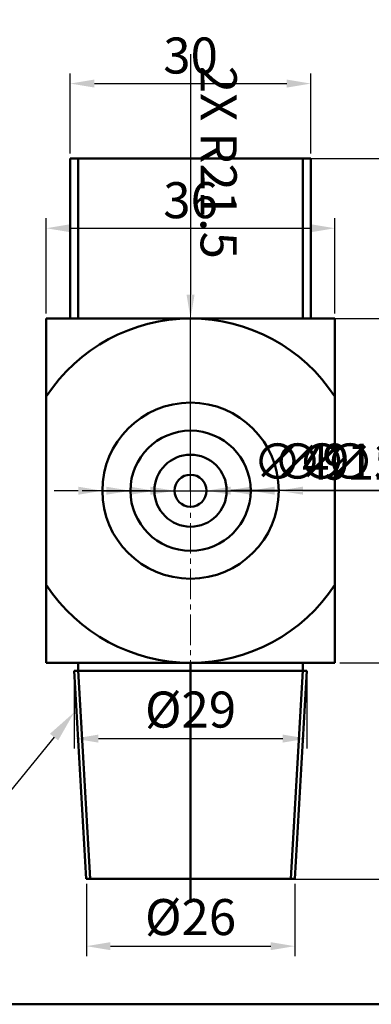
# Model space of a CAD drawing. Units: millimetres. Extents: x 418 to 773, y -46 to 294.
# Tile 3 of 7: x 565 to 609, y -46 to 77. Entities that reach past the tile are written whole.
import ezdxf
from ezdxf import colors
from ezdxf.entities.mleader import LeaderData, LeaderLine
from ezdxf.math import Vec2, Vec3

# ---------------------------------------------------------------- set-up
doc = ezdxf.new("R2010")
doc.units = ezdxf.units.MM
doc.header["$LTSCALE"] = 0.2
doc.linetypes.add('CENTER2', pattern=[28.575, 19.05, -3.175, 3.175, -3.175])
for name, color, linetype, lineweight in [('M-CNTR', 1, 'CENTER2', 18), ('M-DIMS', 2, 'Continuous', 25), ('M-OUTL', 7, 'Continuous', 50), ('M-TEXT', 3, 'Continuous', 25), ('M-TTLB', 7, 'Continuous', 50)]:
    doc.layers.add(name, color=color, linetype=linetype, lineweight=lineweight)
doc.styles.get("Standard").update_dxf_attribs({"font": 'arial.ttf'})
doc.dimstyles.new('ISO-25', dxfattribs={"dimtxt": 4.5, "dimasz": 3, "dimexe": 1.25, "dimexo": 0.625, "dimtad": 1, "dimdec": 1, "dimtxsty": 'Standard', "dimcen": 2.5, "dimadec": 0, "dimazin": 0, "dimtfac": 1, "dimtdec": 1, "dimtmove": 0, "dimatfit": 3, "dimfxl": 1, "dimarcsym": 0})

# ---------------------------------------------------------------- blocks, each defined once
blk = doc.blocks.new('*D87')
at = {"layer": 'Defpoints', "color": 0, "ltscale": 0.2, "transparency": 16777216}
for p in [(601.02, 68.54), (571.02, 59.18), (601.02, 59.18)]:
    blk.add_point(p, dxfattribs=at)
at = {"layer": 'M-DIMS', "color": 0, "lineweight": -2, "ltscale": 0.2, "transparency": 16777216}
for p, q in [((571.02, 59.81), (571.02, 69.79)), ((601.02, 59.81), (601.02, 69.79)), ((574.02, 68.54), (598.02, 68.54))]:
    blk.add_line(p, q, dxfattribs=at)
at = {"layer": 'M-DIMS', "color": 0, "ltscale": 0.2, "transparency": 16777216}
for points in [[(574.02, 69.04), (574.02, 68.04), (571.02, 68.54)], [(598.02, 69.04), (598.02, 68.04), (601.02, 68.54)]]:
    blk.add_solid(points, dxfattribs=at)
at = {"layer": 'M-DIMS', "color": 0, "ltscale": 0.2, "transparency": 16777216, "insert": (586.02, 71.46), "char_height": 4.5, "attachment_point": 5}
blk.add_mtext('30', dxfattribs=at)
blk = doc.blocks.new('*D88')
at = {"layer": 'Defpoints', "color": 0, "ltscale": 0.2, "transparency": 16777216}
for p in [(604.02, 50.47), (568.02, 39.18), (604.02, 39.18)]:
    blk.add_point(p, dxfattribs=at)
at = {"layer": 'M-DIMS', "color": 0, "lineweight": -2, "ltscale": 0.2, "transparency": 16777216}
for p, q in [((568.02, 39.81), (568.02, 51.72)), ((604.02, 39.81), (604.02, 51.72)), ((571.02, 50.47), (601.02, 50.47))]:
    blk.add_line(p, q, dxfattribs=at)
at = {"layer": 'M-DIMS', "color": 0, "ltscale": 0.2, "transparency": 16777216}
for points in [[(571.02, 50.97), (571.02, 49.97), (568.02, 50.47)], [(601.02, 50.97), (601.02, 49.97), (604.02, 50.47)]]:
    blk.add_solid(points, dxfattribs=at)
at = {"layer": 'M-DIMS', "color": 0, "ltscale": 0.2, "transparency": 16777216, "insert": (586.02, 53.39), "char_height": 4.5, "attachment_point": 5}
blk.add_mtext('36', dxfattribs=at)
blk = doc.blocks.new('*D90')
at = {"layer": 'Defpoints', "color": 0, "ltscale": 0.2, "transparency": 16777216}
for p in [(600.02, 59.18), (601.02, 39.18), (620.1, 39.18)]:
    blk.add_point(p, dxfattribs=at)
at = {"layer": 'M-DIMS', "color": 0, "lineweight": -2, "ltscale": 0.2, "transparency": 16777216}
for p, q in [((600.64, 59.18), (621.35, 59.18)), ((620.1, 56.18), (620.1, 42.18)), ((601.64, 39.18), (621.35, 39.18))]:
    blk.add_line(p, q, dxfattribs=at)
at = {"layer": 'M-DIMS', "color": 0, "ltscale": 0.2, "transparency": 16777216}
for points in [[(619.6, 56.18), (620.6, 56.18), (620.1, 59.18)], [(619.6, 42.18), (620.6, 42.18), (620.1, 39.18)]]:
    blk.add_solid(points, dxfattribs=at)
at = {"layer": 'M-DIMS', "color": 0, "ltscale": 0.2, "transparency": 16777216, "insert": (617.18, 49.18), "char_height": 4.5, "attachment_point": 5, "rotation": 90}
blk.add_mtext('20', dxfattribs=at)
blk = doc.blocks.new('*D91')
at = {"layer": 'Defpoints', "color": 0, "ltscale": 0.2, "transparency": 16777216}
for p in [(611.5, 39.18), (604.02, -3.82), (620.1, -3.82)]:
    blk.add_point(p, dxfattribs=at)
at = {"layer": 'M-DIMS', "color": 0, "lineweight": -2, "ltscale": 0.2, "transparency": 16777216}
for p, q in [((612.12, 39.18), (621.35, 39.18)), ((620.1, 36.18), (620.1, -0.82)), ((604.64, -3.82), (621.35, -3.82))]:
    blk.add_line(p, q, dxfattribs=at)
at = {"layer": 'M-DIMS', "color": 0, "ltscale": 0.2, "transparency": 16777216}
for points in [[(619.6, 36.18), (620.6, 36.18), (620.1, 39.18)], [(619.6, -0.82), (620.6, -0.82), (620.1, -3.82)]]:
    blk.add_solid(points, dxfattribs=at)
at = {"layer": 'M-DIMS', "color": 0, "ltscale": 0.2, "transparency": 16777216, "insert": (617.18, 17.68), "char_height": 4.5, "attachment_point": 5, "rotation": 90}
blk.add_mtext('43', dxfattribs=at)
blk = doc.blocks.new('*D92')
at = {"layer": 'Defpoints', "color": 0, "ltscale": 0.2, "transparency": 16777216}
for p in [(608.93, -3.82), (592.52, -30.82), (620.1, -30.82)]:
    blk.add_point(p, dxfattribs=at)
at = {"layer": 'M-DIMS', "color": 0, "lineweight": -2, "ltscale": 0.2, "transparency": 16777216}
for p, q in [((609.56, -3.82), (621.35, -3.82)), ((620.1, -6.82), (620.1, -27.82)), ((593.14, -30.82), (621.35, -30.82))]:
    blk.add_line(p, q, dxfattribs=at)
at = {"layer": 'M-DIMS', "color": 0, "ltscale": 0.2, "transparency": 16777216}
for points in [[(619.6, -6.82), (620.6, -6.82), (620.1, -3.82)], [(619.6, -27.82), (620.6, -27.82), (620.1, -30.82)]]:
    blk.add_solid(points, dxfattribs=at)
at = {"layer": 'M-DIMS', "color": 0, "ltscale": 0.2, "transparency": 16777216, "insert": (617.22, -17.32), "char_height": 4.5, "attachment_point": 5, "rotation": 90}
blk.add_mtext('27', dxfattribs=at)
blk = doc.blocks.new('*D93')
at = {"layer": 'Defpoints', "color": 0, "ltscale": 0.2, "transparency": 16777216}
for p in [(571.52, -4.82), (600.52, -4.82), (600.52, -13.28)]:
    blk.add_point(p, dxfattribs=at)
at = {"layer": 'M-DIMS', "color": 0, "lineweight": -2, "ltscale": 0.2, "transparency": 16777216}
for p, q in [((571.52, -5.44), (571.52, -14.53)), ((600.52, -5.44), (600.52, -14.53)), ((574.52, -13.28), (597.52, -13.28))]:
    blk.add_line(p, q, dxfattribs=at)
at = {"layer": 'M-DIMS', "color": 0, "ltscale": 0.2, "transparency": 16777216}
for points in [[(574.52, -12.78), (574.52, -13.78), (571.52, -13.28)], [(597.52, -12.78), (597.52, -13.78), (600.52, -13.28)]]:
    blk.add_solid(points, dxfattribs=at)
at = {"layer": 'M-DIMS', "color": 0, "ltscale": 0.2, "transparency": 16777216, "insert": (586.02, -10.24), "char_height": 4.5, "attachment_point": 5}
blk.add_mtext('%%C29', dxfattribs=at)
blk = doc.blocks.new('*D94')
at = {"layer": 'Defpoints', "color": 0, "ltscale": 0.2, "transparency": 16777216}
for p in [(573.02, -30.82), (599.02, -30.82), (599.02, -39.21)]:
    blk.add_point(p, dxfattribs=at)
at = {"layer": 'M-DIMS', "color": 0, "lineweight": -2, "ltscale": 0.2, "transparency": 16777216}
for p, q in [((573.02, -31.44), (573.02, -40.46)), ((599.02, -31.44), (599.02, -40.46)), ((576.02, -39.21), (596.02, -39.21))]:
    blk.add_line(p, q, dxfattribs=at)
at = {"layer": 'M-DIMS', "color": 0, "ltscale": 0.2, "transparency": 16777216}
for points in [[(576.02, -38.71), (576.02, -39.71), (573.02, -39.21)], [(596.02, -38.71), (596.02, -39.71), (599.02, -39.21)]]:
    blk.add_solid(points, dxfattribs=at)
at = {"layer": 'M-DIMS', "color": 0, "ltscale": 0.2, "transparency": 16777216, "insert": (586.02, -36.16), "char_height": 4.5, "attachment_point": 5}
blk.add_mtext('%%C26', dxfattribs=at)
blk = doc.blocks.new('*U95')
at = {"layer": 'M-CNTR', "color": 0, "transparency": 16777216}
blk.add_line((0, -25), (0, 47.23), dxfattribs=at)
blk = doc.blocks.new('*D101')
at = {"layer": 'Defpoints', "color": 0, "ltscale": 0.2, "transparency": 16777216}
for p in [(586.02, 39.18), (586.02, 17.68)]:
    blk.add_point(p, dxfattribs=at)
at = {"layer": 'M-DIMS', "color": 0, "lineweight": -2, "ltscale": 0.2, "transparency": 16777216}
for p, q in [((586.02, 72.21), (586.02, 42.18)), ((586.02, 17.68), (586.02, 39.18))]:
    blk.add_line(p, q, dxfattribs=at)
at = {"layer": 'M-DIMS', "color": 0, "ltscale": 0.2, "transparency": 16777216}
blk.add_solid([(586.52, 42.18), (585.52, 42.18), (586.02, 39.18)], dxfattribs=at)
at = {"layer": 'M-DIMS', "color": 0, "ltscale": 0.2, "transparency": 16777216, "insert": (588.94, 58.7), "char_height": 4.5, "attachment_point": 5, "rotation": 270.0004}
blk.add_mtext('2X R21.5', dxfattribs=at)
blk = doc.blocks.new('*D102')
at = {"layer": 'Defpoints', "color": 0, "ltscale": 0.2, "transparency": 16777216}
for p in [(575.02, 17.68), (597.02, 17.68)]:
    blk.add_point(p, dxfattribs=at)
at = {"layer": 'M-DIMS', "color": 0, "lineweight": -2, "ltscale": 0.2, "transparency": 16777216}
for p, q in [((572.02, 17.68), (569.02, 17.68)), ((575.02, 17.68), (597.02, 17.68)), ((615.56, 17.69), (600.02, 17.68))]:
    blk.add_line(p, q, dxfattribs=at)
at = {"layer": 'M-DIMS', "color": 0, "ltscale": 0.2, "transparency": 16777216}
for points in [[(572.02, 18.18), (572.02, 17.18), (575.02, 17.68)], [(600.02, 18.19), (600.02, 17.19), (597.02, 17.68)]]:
    blk.add_solid(points, dxfattribs=at)
at = {"layer": 'M-DIMS', "color": 0, "ltscale": 0.2, "transparency": 16777216, "insert": (609.29, 20.73), "char_height": 4.5, "attachment_point": 5, "rotation": 0.0004}
blk.add_mtext('∅22', dxfattribs=at)
blk = doc.blocks.new('*D103')
at = {"layer": 'Defpoints', "color": 0, "ltscale": 0.2, "transparency": 16777216}
for p in [(578.52, 17.68), (593.52, 17.69)]:
    blk.add_point(p, dxfattribs=at)
at = {"layer": 'M-DIMS', "color": 0, "lineweight": -2, "ltscale": 0.2, "transparency": 16777216}
for p, q in [((575.52, 17.68), (572.52, 17.68)), ((578.52, 17.68), (593.52, 17.69)), ((612.14, 17.69), (596.52, 17.69))]:
    blk.add_line(p, q, dxfattribs=at)
at = {"layer": 'M-DIMS', "color": 0, "ltscale": 0.2, "transparency": 16777216}
for points in [[(575.52, 18.18), (575.52, 17.18), (578.52, 17.68)], [(596.52, 18.19), (596.52, 17.19), (593.52, 17.69)]]:
    blk.add_solid(points, dxfattribs=at)
at = {"layer": 'M-DIMS', "color": 0, "ltscale": 0.2, "transparency": 16777216, "insert": (605.83, 20.73), "char_height": 4.5, "attachment_point": 5, "rotation": 0.0006}
blk.add_mtext('∅15', dxfattribs=at)
blk = doc.blocks.new('*D104')
at = {"layer": 'Defpoints', "color": 0, "ltscale": 0.2, "transparency": 16777216}
for p in [(581.52, 17.68), (590.52, 17.68)]:
    blk.add_point(p, dxfattribs=at)
at = {"layer": 'M-DIMS', "color": 0, "lineweight": -2, "ltscale": 0.2, "transparency": 16777216}
for p, q in [((578.52, 17.68), (575.52, 17.68)), ((581.52, 17.68), (590.52, 17.68)), ((605.62, 17.69), (593.52, 17.68))]:
    blk.add_line(p, q, dxfattribs=at)
at = {"layer": 'M-DIMS', "color": 0, "ltscale": 0.2, "transparency": 16777216}
for points in [[(578.52, 18.18), (578.52, 17.18), (581.52, 17.68)], [(593.52, 18.19), (593.52, 17.19), (590.52, 17.68)]]:
    blk.add_solid(points, dxfattribs=at)
at = {"layer": 'M-DIMS', "color": 0, "ltscale": 0.2, "transparency": 16777216, "insert": (601.07, 20.73), "char_height": 4.5, "attachment_point": 5, "rotation": 0.001}
blk.add_mtext('∅9', dxfattribs=at)
blk = doc.blocks.new('*D105')
at = {"layer": 'Defpoints', "color": 0, "ltscale": 0.2, "transparency": 16777216}
for p in [(584.02, 17.68), (588.02, 17.69)]:
    blk.add_point(p, dxfattribs=at)
at = {"layer": 'M-DIMS', "color": 0, "lineweight": -2, "ltscale": 0.2, "transparency": 16777216}
for p, q in [((581.02, 17.68), (578.02, 17.68)), ((584.02, 17.68), (588.02, 17.69)), ((603.09, 17.69), (591.02, 17.69))]:
    blk.add_line(p, q, dxfattribs=at)
at = {"layer": 'M-DIMS', "color": 0, "ltscale": 0.2, "transparency": 16777216}
for points in [[(581.02, 18.18), (581.02, 17.18), (584.02, 17.68)], [(591.02, 18.19), (591.02, 17.19), (588.02, 17.69)]]:
    blk.add_solid(points, dxfattribs=at)
at = {"layer": 'M-DIMS', "color": 0, "ltscale": 0.2, "transparency": 16777216, "insert": (598.56, 20.73), "char_height": 4.5, "attachment_point": 5, "rotation": 0.0024}
blk.add_mtext('∅4', dxfattribs=at)

msp = doc.modelspace()

# ---------------------------------------------------------------- linework, layer by layer
at = {"layer": 'M-OUTL', "ltscale": 0.2}
for p, q in [((571.0171, 59.1849), (601.0171, 59.1849)), ((571.0171, 39.1849), (571.0171, 59.1849)), ((572.0171, 39.1849), (572.0171, 59.1849)), ((600.0171, 59.1849), (600.0171, 39.1849)), ((601.0171, 59.1849), (601.0171, 39.1849)), ((586.0171, 39.1849), (568.0171, 39.1849)), ((568.0171, 39.1849), (568.0171, -3.8151)), ((601.0171, 39.1849), (571.0171, 39.1849)), ((604.0171, 39.1849), (601.0171, 39.1849)), ((604.0171, -3.8151), (604.0171, 39.1849)), ((568.0171, -3.8151), (604.0171, -3.8151)), ((571.5171, -4.8151), (600.5171, -4.8151)), ((571.5171, -4.8151), (573.0171, -30.8151)), ((572.0163, -4.7863), (573.5163, -30.7863)), ((572.0171, -4.8151), (572.0171, -3.8151)), ((586.0171, -3.8151), (600.5171, -3.8151)), ((586.0171, -3.8151), (586.0171, -33.7843)), ((600.018, -4.7863), (598.518, -30.7863)), ((599.0171, -30.8151), (600.5171, -4.8151)), ((600.018, -4.7863), (600.018, -3.8151)), ((573.0171, -30.8151), (586.0171, -30.8151)), ((586.0171, -30.8151), (599.0171, -30.8151))]:
    msp.add_line(p, q, dxfattribs=at)
for radius in [11, 7.5, 4.5, 2]:
    msp.add_circle((586.0171, 17.6849), radius, dxfattribs=at)
for start, end in [(33.153408, 146.846592), (213.153408, 326.846592)]:
    msp.add_arc((586.0171, 17.6849), 21.5, start, end, dxfattribs=at)
at = {"layer": 'M-TTLB', "ltscale": 0.2}
msp.add_lwpolyline([(417.9371, 294.4119), (773.2687, 294.4119), (773.2687, -46.4726), (417.9371, -46.4726)], close=True, dxfattribs=at)

# ---------------------------------------------------------------- block references
at = {"layer": 'M-CNTR'}
msp.add_blockref('*U95', (586.0171, 17.6849), dxfattribs=at)

# ---------------------------------------------------------------- dimensions: what is measured, and where the dimension line sits
at = {"layer": 'M-DIMS', "ltscale": 0.2}
for base, p1, p2, picture, middle in [((601.0171, 68.5404), (571.0171, 59.1849), (601.0171, 59.1849), '*D87', (586.0171, 71.4645)), ((604.0171, 50.4662), (568.0171, 39.1849), (604.0171, 39.1849), '*D88', (586.0171, 53.3904))]:
    dim = msp.add_linear_dim(base=base, p1=p1, p2=p2, dimstyle='ISO-25', override={"dimclrd": 0, "dimclre": 0, "dimclrt": 0}, dxfattribs=at)
    dim.commit()
    dim.dimension.update_dxf_attribs({"geometry": picture, "text_midpoint": middle})
dim = msp.add_radius_dim(center=(586.0171, 17.6849), mpoint=(586.017, 39.1849), text='2X <>', dimstyle='ISO-25', override={"dimdec": 1, "dimlfac": 1, "dimrnd": 0, "dimzin": 0, "dimdsep": 46, "dimlunit": 2}, dxfattribs=at)
dim.commit()
dim.dimension.update_dxf_attribs({"geometry": '*D101', "text_midpoint": (588.9394, 58.6976)})
for base, p1, p2, picture, middle in [((620.1049, 39.1849), (600.0171, 59.1849), (601.0171, 39.1849), '*D90', (617.1824, 49.1849)), ((620.1049, -3.8151), (611.4985, 39.1849), (604.0171, -3.8151), '*D91', (617.1808, 17.6849)), ((620.1049, -30.8151), (608.9306, -3.8151), (592.5171, -30.8151), '*D92', (617.2207, -17.3151))]:
    dim = msp.add_linear_dim(base=base, p1=p1, p2=p2, angle=90, dimstyle='ISO-25', override={"dimclrd": 0, "dimclre": 0, "dimclrt": 0}, dxfattribs=at)
    dim.commit()
    dim.dimension.update_dxf_attribs({"geometry": picture, "text_midpoint": middle})
for p1, p2, picture, middle in [((575.0171, 17.6848), (597.0171, 17.685), '*D102', (609.2902, 17.6851)), ((578.5171, 17.6848), (593.5171, 17.685), '*D103', (605.8301, 17.6851))]:
    dim = msp.add_diameter_dim_2p(p1=p1, p2=p2, dimstyle='ISO-25', override={"dimdec": 0, "dimlfac": 1, "dimrnd": 0, "dimzin": 0, "dimdsep": 46, "dimlunit": 2}, dxfattribs=at)
    dim.commit()
    dim.dimension.update_dxf_attribs({"geometry": picture, "text_midpoint": middle})
for p1, p2, picture, middle in [((581.5171, 17.6848), (590.5171, 17.685), '*D104', (601.0697, 17.6852)), ((584.0171, 17.6848), (588.0171, 17.685), '*D105', (598.5559, 17.6854))]:
    dim = msp.add_diameter_dim_2p(p1=p1, p2=p2, dimstyle='ISO-25', override={"dimdec": 0, "dimlfac": 1, "dimrnd": 0, "dimzin": 0, "dimdsep": 46, "dimlunit": 2}, dxfattribs=at)
    dim.commit()
    dim.dimension.update_dxf_attribs({"geometry": picture, "text_midpoint": middle, "dimtype": 163})
for base, p1, p2, picture, middle in [((600.5171, -13.2848), (571.5171, -4.8151), (600.5171, -4.8151), '*D93', (586.0171, -10.2364)), ((599.0171, -39.2062), (573.0171, -30.8151), (599.0171, -30.8151), '*D94', (586.0171, -36.1578))]:
    dim = msp.add_linear_dim(base=base, p1=p1, p2=p2, text='%%C<>', dimstyle='ISO-25', override={"dimclrd": 0, "dimclre": 0, "dimclrt": 0}, dxfattribs=at)
    dim.commit()
    dim.dimension.update_dxf_attribs({"geometry": picture, "text_midpoint": middle})

# ---------------------------------------------------------------- leaders
at = {"layer": 'M-TEXT', "ltscale": 0.2}
ml = msp.add_multileader_mtext('Standard', dxfattribs=at)
ml.set_content('1', color=256)
ml.set_leader_properties()
ml.build(insert=Vec2(0, 0))
ctx = ml.context
ctx.base_point, ctx.char_height, ctx.plane_origin = Vec3(532.8405, -38.2871), 10, Vec3(571.5171, -9.9875)
ctx.text_align_type = 2
notes = []
notes.append((ctx, [(0, (1, 1, 0), (548.5239, -38.2871), (-1, 0), 8, [(0, [(571.5171, -9.9875)], 0, [])])]))
ctx.mtext.insert, ctx.mtext.alignment, ctx.mtext.flow_direction = Vec3(538.5239, -33.2871), 3, 5
for ctx, leaders in notes:
    for number, flags, end, landing, length, lines in leaders:
        leader = LeaderData()
        leader.index, (leader.has_last_leader_line, leader.has_dogleg_vector, leader.attachment_direction) = number, flags
        leader.last_leader_point, leader.dogleg_vector, leader.dogleg_length = Vec3(end), Vec3(landing), length
        for number, points, colour, breaks in lines:
            line = LeaderLine()
            line.index, line.vertices, line.color, line.breaks = number, Vec3.list(points), colors.encode_raw_color(colour), breaks
            leader.lines.append(line)
        ctx.leaders.append(leader)

doc.saveas('drawing.dxf')
